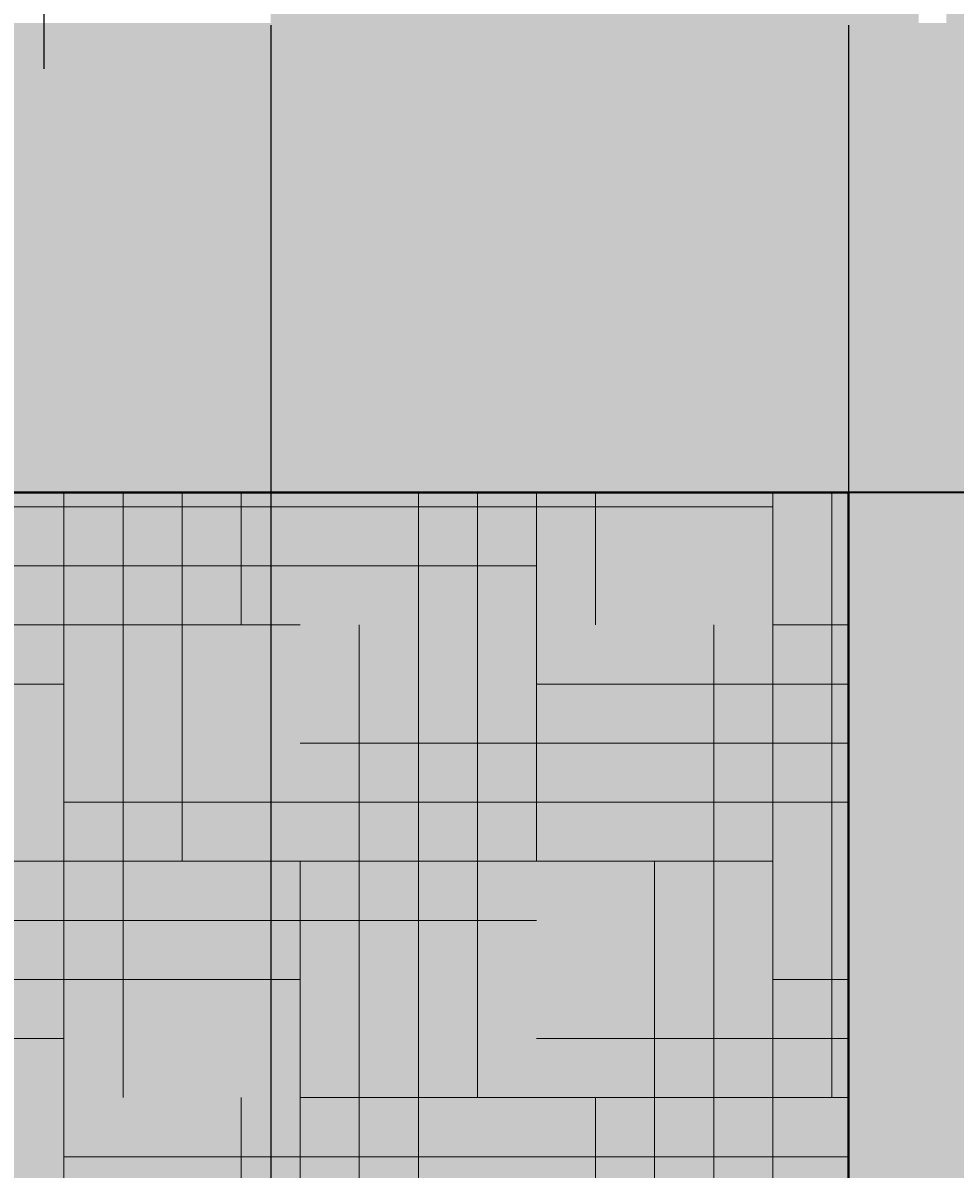
# Model space of a CAD drawing. Units: feet. Extents: x 2695 to 2912, y 795 to 1139.
# Tile 15 of 83: x 2748 to 2774, y 906 to 937. Entities that reach past the tile are written whole.
import ezdxf

# ---------------------------------------------------------------- set-up
doc = ezdxf.new("R2010")
doc.units = ezdxf.units.FT
for name, color, linetype, lineweight in [('A-ANNO-DIMS', 2, 'Continuous', 18), ('A-ELEV', 7, 'Continuous', 35), ('A-ELEV-PATT', 252, 'Continuous', 13), ('A-GLAZ', 4, 'Continuous', 25)]:
    doc.layers.add(name, color=color, linetype=linetype, lineweight=lineweight)
doc.styles.get("Standard").update_dxf_attribs({"font": 'arial.ttf'})
doc.dimstyles.get("Standard").update_dxf_attribs({"dimtxt": 0.18, "dimasz": 0.18, "dimexe": 0.18, "dimexo": 0.0625, "dimgap": 0.09, "dimtad": 0, "dimtih": 1, "dimtoh": 1, "dimdec": 1, "dimzin": 0, "dimdsep": 46, "dimlunit": 3, "dimtxsty": 'Standard', "dimcen": 0.09, "dimadec": 0, "dimazin": 0, "dimtfac": 1, "dimtdec": 1, "dimtofl": 0, "dimtmove": 0, "dimatfit": 3, "dimfxl": 1, "dimtolj": 1, "dimtzin": 0, "dimarcsym": 0})

# ---------------------------------------------------------------- blocks, each defined once
blk = doc.blocks.new('*D24')
at = {"layer": 'A-ANNO-DIMS', "color": 0, "lineweight": -2, "transparency": 16777216}
for p, q in [((2730.708, 936.868), (2730.708, 794.976)), ((2755.112, 936.868), (2755.112, 794.976)), ((2730.888, 795.156), (2742.446, 795.156)), ((2754.932, 795.156), (2743.375, 795.156))]:
    blk.add_line(p, q, dxfattribs=at)
at = {"layer": 'A-ANNO-DIMS', "color": 0, "transparency": 16777216}
for points in [[(2730.888, 795.186), (2730.888, 795.126), (2730.708, 795.156)], [(2754.932, 795.186), (2754.932, 795.126), (2755.112, 795.156)]]:
    blk.add_solid(points, dxfattribs=at)
at = {"layer": 'Defpoints', "color": 0, "transparency": 16777216}
for p in [(2730.708, 936.931), (2755.112, 936.931), (2755.112, 795.156)]:
    blk.add_point(p, dxfattribs=at)
at = {"layer": 'A-ANNO-DIMS', "color": 0, "transparency": 16777216, "insert": (2742.91, 795.156), "char_height": 0.18, "attachment_point": 5}
blk.add_mtext('\\A1;24.404', dxfattribs=at)
blk = doc.blocks.new('*D25')
at = {"layer": 'A-ANNO-DIMS', "color": 0, "lineweight": -2, "transparency": 16777216}
for p, q in [((2755.112, 936.868), (2755.112, 794.976)), ((2770.636, 936.868), (2770.636, 794.976)), ((2755.292, 795.156), (2762.419, 795.156)), ((2770.456, 795.156), (2763.329, 795.156))]:
    blk.add_line(p, q, dxfattribs=at)
at = {"layer": 'A-ANNO-DIMS', "color": 0, "transparency": 16777216}
for points in [[(2755.292, 795.186), (2755.292, 795.126), (2755.112, 795.156)], [(2770.456, 795.186), (2770.456, 795.126), (2770.636, 795.156)]]:
    blk.add_solid(points, dxfattribs=at)
at = {"layer": 'Defpoints', "color": 0, "transparency": 16777216}
for p in [(2755.112, 936.931), (2770.636, 936.931), (2770.636, 795.156)]:
    blk.add_point(p, dxfattribs=at)
at = {"layer": 'A-ANNO-DIMS', "color": 0, "transparency": 16777216, "insert": (2762.874, 795.156), "char_height": 0.18, "attachment_point": 5}
blk.add_mtext('\\A1;15.524', dxfattribs=at)

msp = doc.modelspace()

# ---------------------------------------------------------------- hatches: boundary and pattern name
at = {"layer": 'A-ELEV-PATT'}
h = msp.add_hatch(color=256, dxfattribs=at)
h.set_gradient(color1=(255, 255, 255), tint=1)
h.paths.add_polyline_path([(2770.6361, 1122.9306), (2710.6361, 1122.9306), (2710.6361, 1118.4096), (2770.6361, 1118.4096)])
h.paths.add_polyline_path([(2890.6361, 1107.8588), (2770.6361, 1107.8588), (2770.6361, 1103.3378), (2890.6361, 1103.3378)])
h.paths.add_polyline_path([(2890.6361, 1062.9306), (2710.6361, 1062.9306), (2710.6361, 1056.9306), (2710.6361, 936.9306), (2710.6361, 924.3105), (2716.5358, 924.3105), (2890.6361, 924.3105), (2890.6361, 936.9306), (2715.8852, 936.9306), (2715.8852, 1050.3105), (2890.6361, 1050.3105)])
h.paths.add_polyline_path([(2716.5358, 924.3105), (2710.6361, 924.3105), (2710.6361, 810.9306), (2716.5358, 810.9306)])
h = msp.add_hatch(color=256, dxfattribs=at)
h.set_gradient(color1=(147, 149, 152), color2=(147, 149, 152), tint=1)
h.paths.add_polyline_path([(2770.6361, 1118.4096), (2710.6361, 1118.4096), (2710.6361, 1062.9306), (2770.6361, 1062.9306)])
h.paths.add_polyline_path([(2890.6361, 1103.3378), (2770.6361, 1103.3378), (2770.6361, 1062.9306), (2890.6361, 1062.9306)])
h.paths.add_polyline_path([(2730.7081, 1048.1052), (2755.1125, 1048.1052), (2755.1125, 936.9306), (2770.6361, 936.9306), (2770.6361, 1050.3105), (2715.8852, 1050.3105), (2715.8852, 936.9306), (2730.7081, 936.9306)])
h.paths.add_polyline_path([(2890.6361, 1050.3105), (2770.6361, 1050.3105), (2770.6361, 971.9673), (2778.0341, 971.9673), (2778.0341, 1020.8235), (2843.575, 1020.8235), (2843.575, 971.9673), (2890.6361, 971.9673)])
h.paths.add_polyline_path([(2888.1882, 970.7156), (2843.575, 970.7156), (2843.575, 964.8267), (2888.1882, 964.8267)])
h.paths.add_polyline_path([(2888.1882, 964.1328), (2843.575, 964.1328), (2843.575, 956.614), (2888.1882, 956.614)])
h.paths.add_polyline_path([(2888.1882, 955.9202), (2843.575, 955.9202), (2843.575, 949.2892), (2888.1882, 949.2892)])
h.paths.add_polyline_path([(2888.1882, 948.5954), (2843.575, 948.5954), (2843.575, 941.3507), (2888.1882, 941.3507)])
h.paths.add_polyline_path([(2888.1882, 940.6569), (2843.575, 940.6569), (2843.575, 936.9306), (2888.1882, 936.9306)])
h.paths.add_polyline_path([(2890.6361, 970.7156), (2888.9368, 970.7156), (2888.9368, 964.8267), (2890.6361, 964.8267)])
h.paths.add_polyline_path([(2890.6361, 964.1328), (2888.9368, 964.1328), (2888.9368, 956.614), (2890.6361, 956.614)])
h.paths.add_polyline_path([(2890.6361, 955.9202), (2888.9368, 955.9202), (2888.9368, 949.2892), (2890.6361, 949.2892)])
h.paths.add_polyline_path([(2890.6361, 940.6569), (2888.9368, 940.6569), (2888.9368, 936.9306), (2890.6361, 936.9306)])
h.paths.add_polyline_path([(2890.6361, 948.5954), (2888.9368, 948.5954), (2888.9368, 941.3507), (2890.6361, 941.3507)])
h.paths.add_polyline_path([(2772.5216, 970.7156), (2770.6361, 970.7156), (2770.6361, 964.8267), (2772.5216, 964.8267)])
h.paths.add_polyline_path([(2772.5216, 964.1328), (2770.6361, 964.1328), (2770.6361, 956.614), (2772.5216, 956.614)])
h.paths.add_polyline_path([(2772.5216, 955.9202), (2770.6361, 955.9202), (2770.6361, 949.2892), (2772.5216, 949.2892)])
h.paths.add_polyline_path([(2772.5216, 948.5954), (2770.6361, 948.5954), (2770.6361, 941.3507), (2772.5216, 941.3507)])
h.paths.add_polyline_path([(2772.5216, 940.6569), (2770.6361, 940.6569), (2770.6361, 936.9306), (2772.5216, 936.9306)])
h.paths.add_polyline_path([(2778.0341, 940.6569), (2773.2702, 940.6569), (2773.2702, 936.9306), (2778.0341, 936.9306)])
h.paths.add_polyline_path([(2778.0341, 970.7156), (2773.2702, 970.7156), (2773.2702, 964.8267), (2778.0341, 964.8267)])
h.paths.add_polyline_path([(2778.0341, 964.1328), (2773.2702, 964.1328), (2773.2702, 956.614), (2778.0341, 956.614)])
h.paths.add_polyline_path([(2778.0341, 955.9202), (2773.2702, 955.9202), (2773.2702, 949.2892), (2778.0341, 949.2892)])
h.paths.add_polyline_path([(2778.0341, 948.5954), (2773.2702, 948.5954), (2773.2702, 941.3507), (2778.0341, 941.3507)])
h.paths.add_polyline_path([(2810.0407, 940.6569), (2780.0341, 940.6569), (2780.0341, 936.9306), (2810.0407, 936.9306)])
h.paths.add_polyline_path([(2890.6361, 924.3105), (2770.6361, 924.3105), (2770.6361, 810.9306), (2773.5029, 810.9306), (2773.5029, 905.5143), (2805.9398, 905.5143), (2838.3767, 905.5143), (2838.3767, 810.9306), (2890.6361, 810.9306)])
h = msp.add_hatch(color=256, dxfattribs=at)
h.set_gradient(color1=(255, 255, 255))
h.paths.add_polyline_path([(2770.6361, 924.3105), (2716.5358, 924.3105), (2716.5358, 810.9306), (2770.6361, 810.9306)])
h.paths.add_polyline_path([(2758.1515, 902.577), (2758.1515, 874.8571), (2724.1893, 874.8571), (2724.1893, 902.577)], flags=16)
h.paths.add_polyline_path([(2756.1515, 900.577), (2756.1515, 876.8571), (2726.1893, 876.8571), (2726.1893, 900.577)], flags=0)
h.paths.add_polyline_path([(2740.7302, 900.577), (2741.6105, 900.577), (2741.6105, 876.8571), (2740.7302, 876.8571)], flags=0)
h = msp.add_hatch(dxfattribs=at)
h.set_pattern_fill('HOUND', color=256, style=0)
h.paths.add_polyline_path([(2770.6361, 924.3105), (2716.5358, 924.3105), (2716.5358, 810.9306), (2770.6361, 810.9306)])
h.paths.add_polyline_path([(2724.1893, 874.8571), (2724.1893, 902.577), (2758.1515, 902.577), (2758.1515, 874.8571)], flags=16)
h.paths.add_polyline_path([(2756.1515, 876.8571), (2726.1893, 876.8571), (2726.1893, 900.577), (2756.1515, 900.577)], flags=0)
h.paths.add_polyline_path([(2741.6105, 876.8571), (2740.7302, 876.8571), (2740.7302, 900.577), (2741.6105, 900.577)], flags=0)

# ---------------------------------------------------------------- linework, layer by layer
at = {"layer": 'A-ELEV'}
for p, q in [((2770.6361, 924.3105), (2716.5358, 924.3105)), ((2770.6361, 924.3105), (2770.6361, 810.9306)), ((2770.6361, 810.9306), (2770.6361, 924.3105))]:
    msp.add_line(p, q, dxfattribs=at)
msp.add_lwpolyline([(2890.6361, 936.9306), (2890.6361, 924.3105), (2710.6361, 924.3105), (2710.6361, 936.9306)], dxfattribs=at)
msp.add_lwpolyline([(2716.5358, 924.3105), (2770.6361, 924.3105), (2770.6361, 810.9306), (2716.5358, 810.9306)], close=True, dxfattribs=at)
at = {"layer": 'A-GLAZ'}
msp.add_line((2749.0114, 1048.1052), (2749.0114, 935.6966), dxfattribs=at)

# ---------------------------------------------------------------- dimensions: what is measured, and where the dimension line sits
at = {"layer": 'A-ANNO-DIMS'}
for base, p1, p2, picture, middle in [((2755.1125, 795.1556), (2730.7081, 936.9306), (2755.1125, 936.9306), '*D24', (2742.9103, 795.1556)), ((2770.6361, 795.1556), (2755.1125, 936.9306), (2770.6361, 936.9306), '*D25', (2762.8743, 795.1556))]:
    dim = msp.add_linear_dim(base=base, p1=p1, p2=p2, dimstyle='Standard', override={"dimdec": 3, "dimlfac": 1, "dimrnd": 0, "dimzin": 0, "dimdsep": 46, "dimlunit": 2}, dxfattribs=at)
    dim.commit()
    dim.dimension.update_dxf_attribs({"geometry": picture, "text_midpoint": middle})

doc.saveas('drawing.dxf')
